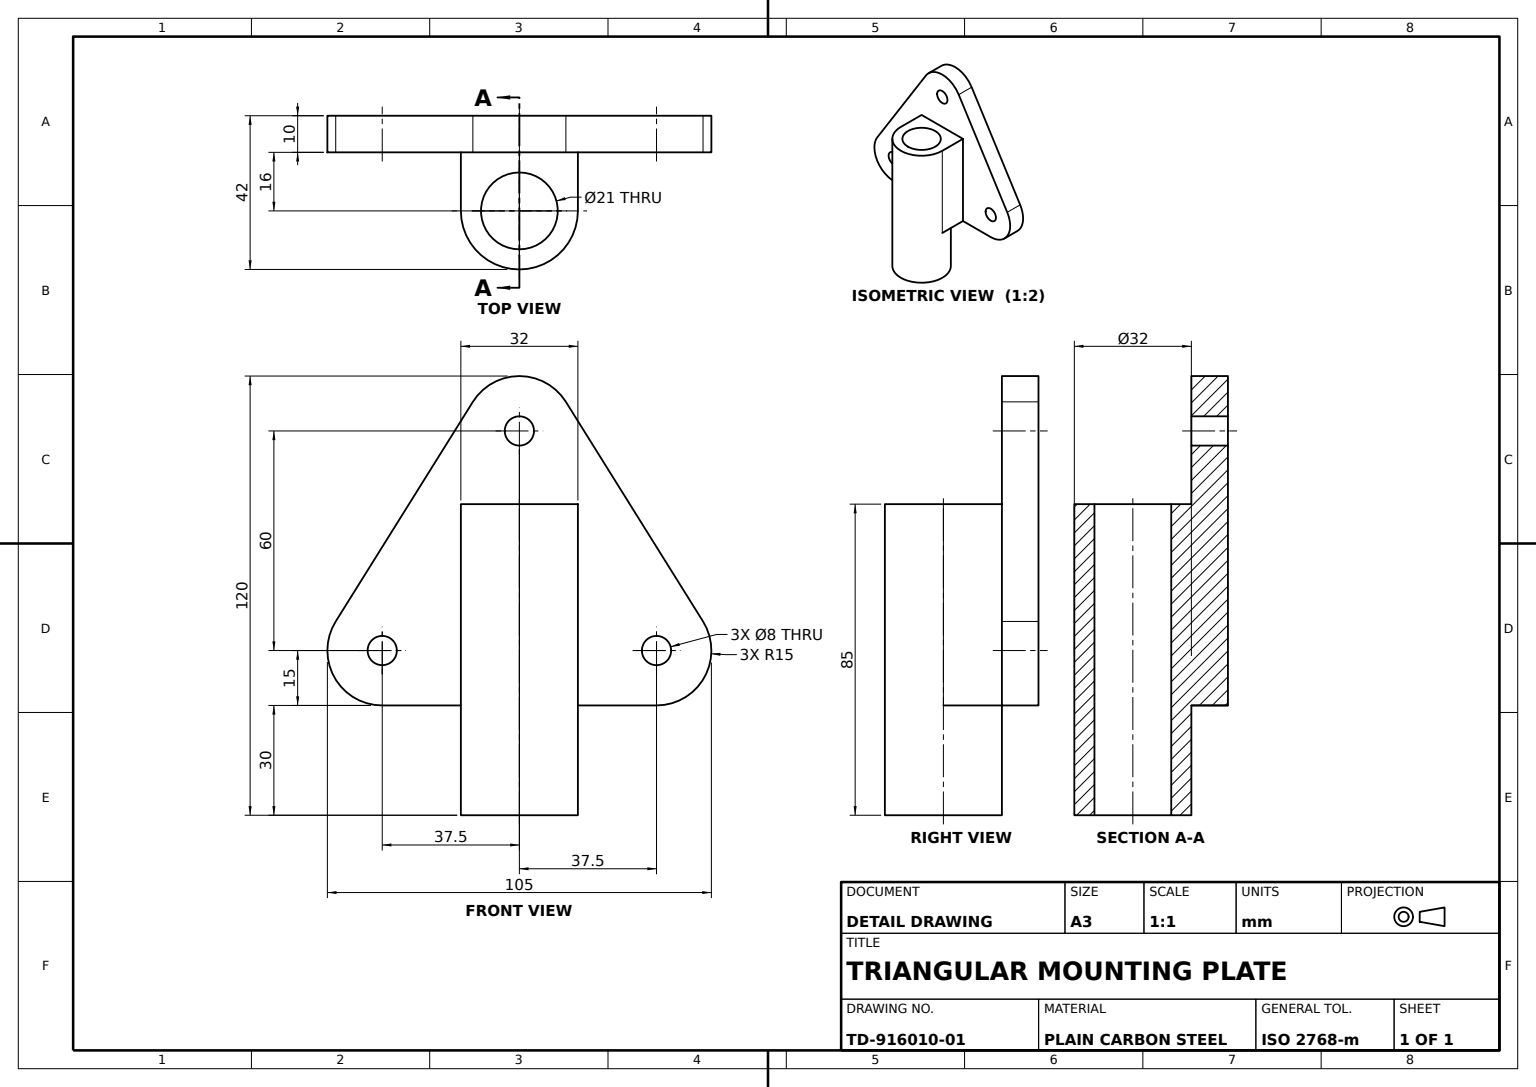
SolidWorks part; units mm, degrees
material "Plain Carbon Steel"
ref_plane "Front Plane" through (0, 0, 0) normal (0, 0, 1) x (1, 0, 0)
ref_plane "Top Plane" through (0, 0, 0) normal (0, 1, 0) x (1, 0, 0)
ref_plane "Right Plane" through (0, 0, 0) normal (1, 0, 0) x (0, 0, -1)
sketch "Base Plate Profile" plane through (0, 0, 0) normal (0, 0, 1) x (1, 0, 0)
  line L0 (0, 0) -> (0, -60)
  line L1 (0, -60) -> (37.5, -60)
  line L2 (0, -60) -> (-37.5, -60)
  line L3 (-50.22, -52.05) -> (-12.72, 7.95)
  line L4 (-37.5, -75) -> (37.5, -75)
  line L5 (12.72, 7.95) -> (50.22, -52.05)
  arc A0 (12.72, 7.95) -> (-12.72, 7.95) centre (0, 0) ccw
  arc A1 (-50.22, -52.05) -> (-37.5, -75) centre (-37.5, -60) ccw
  arc A2 (37.5, -75) -> (50.22, -52.05) centre (37.5, -60) ccw
  dimension "D1" = 15
  dimension "D6" = 15
  dimension "D2" = 60
  dimension "D3" = 37.5
  dimension "D4" = 37.5
extrude "Triangular Base Plate" add sketch "Base Plate Profile" along normal blind 10
sketch "Tube Support Block Profile" plane through (0, -75, 0) normal (0, -1, 0) x (1, 0, 0)
  line L0 (0, 10) -> (0, 20)
  line L1 (-37.5, 10) -> (37.5, 10) construction
  line L2 (0, 20) -> (-16, 20)
  line L3 (-16, 20) -> (-16, 10)
  line L4 (-16, 10) -> (16, 10)
  line L5 (16, 10) -> (16, 20)
  line L6 (16, 20) -> (0, 20)
  line M3 (37.5, 10) -> (-37.5, 10)
  dimension "D1" = 10
  dimension "D2" = 16
  dimension "D3" = 32
extrude "Tube Support Block" add sketch "Tube Support Block Profile" against normal blind 55 contours L2 L3 L0 M3 | L5 L6 L0 M3
sketch "Support Web Profile" plane through (0, -75, 0) normal (0, -1, 0) x (1, 0, 0)
  line L0 (0, 20) -> (0, 26)
  line L1 (16, 20) -> (-16, 20) construction
  line L2 (0, 26) -> (16, 26)
  line L3 (16, 26) -> (16, 20)
  line L4 (16, 20) -> (-16, 20)
  line L5 (-16, 20) -> (-16, 26)
  line L6 (-16, 26) -> (0, 26)
  line M5 (16, 20) -> (-16, 20)
  dimension "D1" = 6
extrude "Support Web" add sketch "Support Web Profile" against normal blind 55 contours L6 L5 L0 M5 | L3 L2 L0 M5
sketch "Tube Profile Ø32" plane through (0, -75, 0) normal (0, -1, 0) x (1, 0, 0)
  line L0 (-16, 26) -> (16, 26) construction
  circle A0 centre (0, 26) radius 16
  dimension "D1" = 32
extrude "Round Tube Ø32" add sketch "Tube Profile Ø32" against normal blind 55
sketch "Tube Extension Profile Ø32" plane through (0, -75, 0) normal (0, -1, 0) x (1, 0, 0)
  circle A0 centre (0, 26) radius 16
  dimension "D1" = 32
extrude "Tube Extension Ø32" add sketch "Tube Extension Profile Ø32" along normal blind 30
sketch "Tube Bore Profile Ø21" plane through (0, -105, 0) normal (0, -1, 0) x (1, 0, 0)
  circle A0 centre (0, 26) radius 10.5
  dimension "D1" = 21
extrude "Tube Bore Ø21" cut sketch "Tube Bore Profile Ø21" against normal blind 85
sketch "Mounting Holes Profile 3xØ8" plane through (0, 0, 10) normal (0, 0, 1) x (1, 0, 0)
  circle A0 centre (0, 0) radius 4
  circle A1 centre (-37.5, -60) radius 4
  circle A2 centre (37.5, -60) radius 4
  dimension "D1" = 8
  dimension "D2" = 8
  dimension "D3" = 8
extrude "Mounting Holes 3xØ8" cut sketch "Mounting Holes Profile 3xØ8" against normal blind 85
